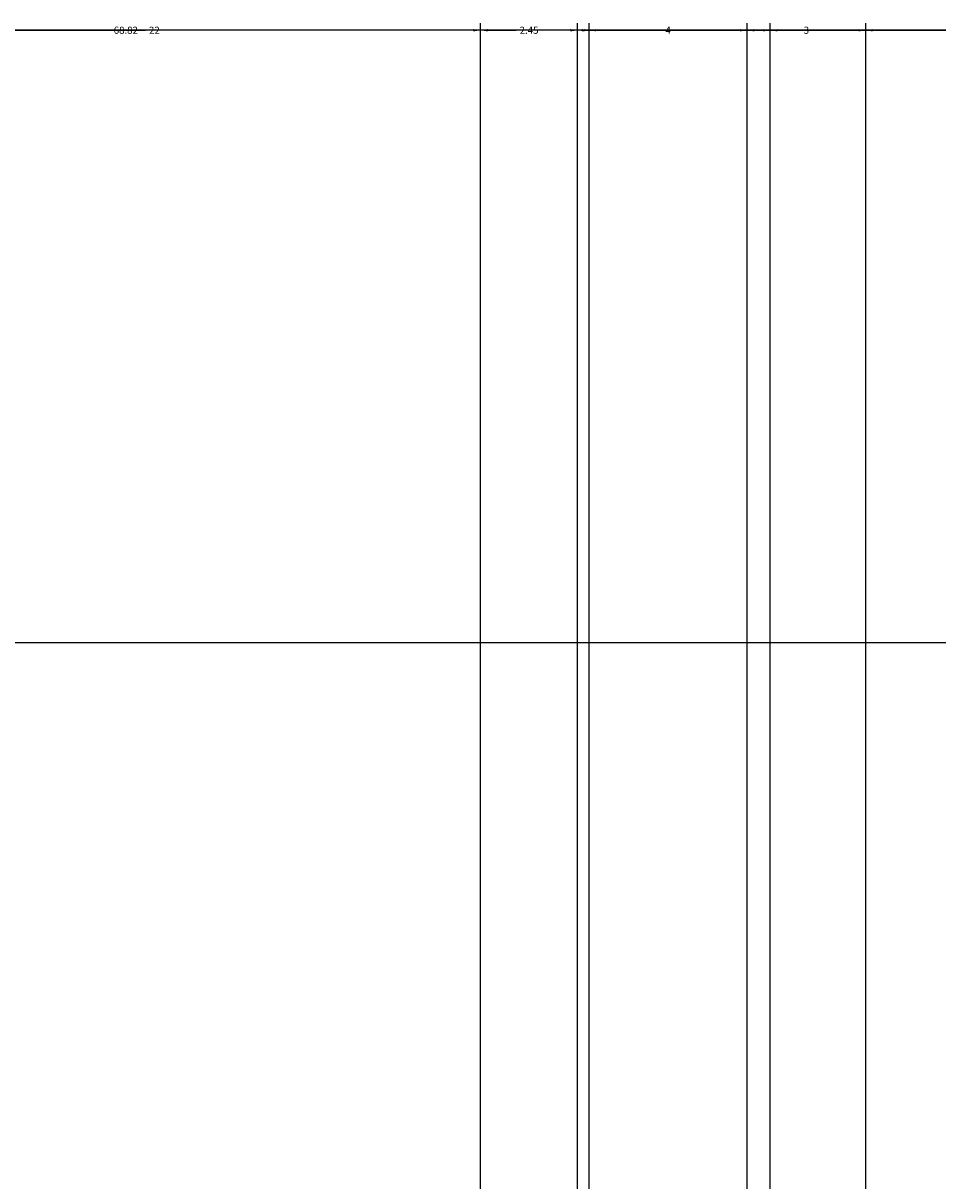
# Model space of a CAD drawing. Units: inches. Extents: x -6 to 289, y -8 to 323.
# Tile 91 of 107: x 150 to 173, y 294 to 323. Entities that reach past the tile are written whole.
import ezdxf

# ---------------------------------------------------------------- set-up
doc = ezdxf.new("R2010")
doc.units = ezdxf.units.IN
doc.header["$MEASUREMENT"] = 0
doc.layers.add('A-ANNO-DIMS', color=2, linetype='Continuous', lineweight=18)
doc.styles.get("Standard").update_dxf_attribs({"font": 'arial.ttf'})
doc.dimstyles.get("Standard").update_dxf_attribs({"dimtxt": 0.18, "dimasz": 0.18, "dimexe": 0.18, "dimexo": 0.0625, "dimgap": 0.09, "dimtad": 0, "dimtih": 1, "dimtoh": 1, "dimdec": 4, "dimzin": 0, "dimdsep": 46, "dimtxsty": 'Standard', "dimcen": 0.09, "dimadec": 0, "dimazin": 0, "dimtfac": 1, "dimtdec": 4, "dimtofl": 0, "dimtmove": 0, "dimatfit": 3, "dimfxl": 1, "dimtolj": 1, "dimtzin": 0, "dimarcsym": 0})

# ---------------------------------------------------------------- blocks, each defined once
blk = doc.blocks.new('*D11')
at = {"layer": 'A-ANNO-DIMS', "color": 0, "lineweight": -2, "transparency": 16777216}
for p, q in [((126.883, 226.717), (126.883, 322.969)), ((168.883, 226.717), (168.883, 322.969)), ((127.063, 322.789), (147.662, 322.789)), ((168.703, 322.789), (148.105, 322.789))]:
    blk.add_line(p, q, dxfattribs=at)
at = {"layer": 'A-ANNO-DIMS', "color": 0, "transparency": 16777216}
for points in [[(127.063, 322.819), (127.063, 322.759), (126.883, 322.789)], [(168.703, 322.819), (168.703, 322.759), (168.883, 322.789)]]:
    blk.add_solid(points, dxfattribs=at)
at = {"layer": 'Defpoints', "color": 0, "transparency": 16777216}
for p in [(168.883, 322.789), (126.883, 226.654), (168.883, 226.654)]:
    blk.add_point(p, dxfattribs=at)
at = {"layer": 'A-ANNO-DIMS', "color": 0, "transparency": 16777216, "insert": (147.883, 322.789), "char_height": 0.18, "attachment_point": 5}
blk.add_mtext('\\A1;42', dxfattribs=at)
blk = doc.blocks.new('*D12')
at = {"layer": 'A-ANNO-DIMS', "color": 0, "lineweight": -2, "transparency": 16777216}
for p, q in [((168.883, 226.717), (168.883, 322.969)), ((188.292, 226.951), (188.292, 322.969)), ((169.063, 322.789), (178.22, 322.789)), ((188.112, 322.789), (178.955, 322.789))]:
    blk.add_line(p, q, dxfattribs=at)
at = {"layer": 'A-ANNO-DIMS', "color": 0, "transparency": 16777216}
for points in [[(169.063, 322.819), (169.063, 322.759), (168.883, 322.789)], [(188.112, 322.819), (188.112, 322.759), (188.292, 322.789)]]:
    blk.add_solid(points, dxfattribs=at)
at = {"layer": 'Defpoints', "color": 0, "transparency": 16777216}
for p in [(188.292, 322.789), (188.292, 226.889), (168.883, 226.654)]:
    blk.add_point(p, dxfattribs=at)
at = {"layer": 'A-ANNO-DIMS', "color": 0, "transparency": 16777216, "insert": (178.588, 322.789), "char_height": 0.18, "attachment_point": 5}
blk.add_mtext('\\A1;19.41', dxfattribs=at)
blk = doc.blocks.new('*D27')
at = {"layer": 'A-ANNO-DIMS', "color": 0, "lineweight": -2, "transparency": 16777216}
for p, q in [((19.226, 307.289), (288.653, 307.289)), ((288.473, 307.109), (288.473, 277.471)), ((288.473, 247.469), (288.473, 277.107)), ((247.226, 247.289), (288.653, 247.289))]:
    blk.add_line(p, q, dxfattribs=at)
at = {"layer": 'A-ANNO-DIMS', "color": 0, "transparency": 16777216}
for points in [[(288.443, 307.109), (288.503, 307.109), (288.473, 307.289)], [(288.443, 247.469), (288.503, 247.469), (288.473, 247.289)]]:
    blk.add_solid(points, dxfattribs=at)
at = {"layer": 'Defpoints', "color": 0, "transparency": 16777216}
for p in [(19.164, 307.289), (288.473, 307.289), (247.164, 247.289)]:
    blk.add_point(p, dxfattribs=at)
at = {"layer": 'A-ANNO-DIMS', "color": 0, "transparency": 16777216, "insert": (288.473, 277.289), "char_height": 0.18, "attachment_point": 5}
blk.add_mtext('\\A1;60', dxfattribs=at)
blk = doc.blocks.new('*D76')
at = {"layer": 'A-ANNO-DIMS', "color": 0, "lineweight": -2, "transparency": 16777216}
for p, q in [((142.296, 51.148), (142.296, 322.969)), ((164.296, 51.148), (164.296, 322.969)), ((142.476, 322.789), (153.076, 322.789)), ((164.116, 322.789), (153.516, 322.789))]:
    blk.add_line(p, q, dxfattribs=at)
at = {"layer": 'A-ANNO-DIMS', "color": 0, "transparency": 16777216}
for points in [[(142.476, 322.819), (142.476, 322.759), (142.296, 322.789)], [(164.116, 322.819), (164.116, 322.759), (164.296, 322.789)]]:
    blk.add_solid(points, dxfattribs=at)
at = {"layer": 'Defpoints', "color": 0, "transparency": 16777216}
for p in [(164.296, 322.789), (142.296, 51.085), (164.296, 51.085)]:
    blk.add_point(p, dxfattribs=at)
at = {"layer": 'A-ANNO-DIMS', "color": 0, "transparency": 16777216, "insert": (153.296, 322.789), "char_height": 0.18, "attachment_point": 5}
blk.add_mtext('\\A1;22', dxfattribs=at)
blk = doc.blocks.new('*D77')
at = {"layer": 'A-ANNO-DIMS', "color": 0, "lineweight": -2, "transparency": 16777216}
for p, q in [((164.296, 51.148), (164.296, 322.969)), ((168.296, 51.148), (168.296, 322.969)), ((164.476, 322.789), (166.144, 322.789)), ((168.116, 322.789), (166.448, 322.789))]:
    blk.add_line(p, q, dxfattribs=at)
at = {"layer": 'A-ANNO-DIMS', "color": 0, "transparency": 16777216}
for points in [[(164.476, 322.819), (164.476, 322.759), (164.296, 322.789)], [(168.116, 322.819), (168.116, 322.759), (168.296, 322.789)]]:
    blk.add_solid(points, dxfattribs=at)
at = {"layer": 'Defpoints', "color": 0, "transparency": 16777216}
for p in [(168.296, 322.789), (164.296, 51.085), (168.296, 51.085)]:
    blk.add_point(p, dxfattribs=at)
at = {"layer": 'A-ANNO-DIMS', "color": 0, "transparency": 16777216, "insert": (166.296, 322.789), "char_height": 0.18, "attachment_point": 5}
blk.add_mtext('\\A1;4', dxfattribs=at)
blk = doc.blocks.new('*D78')
at = {"layer": 'A-ANNO-DIMS', "color": 0, "lineweight": -2, "transparency": 16777216}
for p, q in [((168.296, 51.148), (168.296, 322.969)), ((171.296, 51.148), (171.296, 322.969)), ((168.476, 322.789), (169.647, 322.789)), ((171.116, 322.789), (169.945, 322.789))]:
    blk.add_line(p, q, dxfattribs=at)
at = {"layer": 'A-ANNO-DIMS', "color": 0, "transparency": 16777216}
for points in [[(168.476, 322.819), (168.476, 322.759), (168.296, 322.789)], [(171.116, 322.819), (171.116, 322.759), (171.296, 322.789)]]:
    blk.add_solid(points, dxfattribs=at)
at = {"layer": 'Defpoints', "color": 0, "transparency": 16777216}
for p in [(171.296, 322.789), (168.296, 51.085), (171.296, 51.085)]:
    blk.add_point(p, dxfattribs=at)
at = {"layer": 'A-ANNO-DIMS', "color": 0, "transparency": 16777216, "insert": (169.796, 322.789), "char_height": 0.18, "attachment_point": 5}
blk.add_mtext('\\A1;3', dxfattribs=at)
blk = doc.blocks.new('*D79')
at = {"layer": 'A-ANNO-DIMS', "color": 0, "lineweight": -2, "transparency": 16777216}
for p, q in [((171.296, 118.033), (171.296, 322.969)), ((188.292, 116.842), (188.292, 322.969)), ((171.476, 322.789), (179.339, 322.789)), ((188.112, 322.789), (180.249, 322.789))]:
    blk.add_line(p, q, dxfattribs=at)
at = {"layer": 'A-ANNO-DIMS', "color": 0, "transparency": 16777216}
for points in [[(171.476, 322.819), (171.476, 322.759), (171.296, 322.789)], [(188.112, 322.819), (188.112, 322.759), (188.292, 322.789)]]:
    blk.add_solid(points, dxfattribs=at)
at = {"layer": 'Defpoints', "color": 0, "transparency": 16777216}
for p in [(188.292, 322.789), (171.296, 117.971), (188.292, 116.779)]:
    blk.add_point(p, dxfattribs=at)
at = {"layer": 'A-ANNO-DIMS', "color": 0, "transparency": 16777216, "insert": (179.794, 322.789), "char_height": 0.18, "attachment_point": 5}
blk.add_mtext('\\A1;16.996', dxfattribs=at)
blk = doc.blocks.new('*D94')
at = {"layer": 'A-ANNO-DIMS', "color": 0, "lineweight": -2, "transparency": 16777216}
for p, q in [((118.164, 159.411), (118.164, 322.969)), ((161.552, 159.411), (161.552, 322.969)), ((118.344, 322.789), (139.46, 322.789)), ((161.372, 322.789), (140.256, 322.789))]:
    blk.add_line(p, q, dxfattribs=at)
at = {"layer": 'A-ANNO-DIMS', "color": 0, "transparency": 16777216}
for points in [[(118.344, 322.819), (118.344, 322.759), (118.164, 322.789)], [(161.372, 322.819), (161.372, 322.759), (161.552, 322.789)]]:
    blk.add_solid(points, dxfattribs=at)
at = {"layer": 'Defpoints', "color": 0, "transparency": 16777216}
for p in [(161.552, 322.789), (118.164, 159.348), (161.552, 159.348)]:
    blk.add_point(p, dxfattribs=at)
at = {"layer": 'A-ANNO-DIMS', "color": 0, "transparency": 16777216, "insert": (139.858, 322.789), "char_height": 0.18, "attachment_point": 5}
blk.add_mtext('\\A1;43.39', dxfattribs=at)
blk = doc.blocks.new('*D95')
at = {"layer": 'A-ANNO-DIMS', "color": 0, "lineweight": -2, "transparency": 16777216}
for p, q in [((161.552, 159.411), (161.552, 322.969)), ((164.004, 159.411), (164.004, 322.969)), ((161.732, 322.789), (162.452, 322.789)), ((163.824, 322.789), (163.104, 322.789))]:
    blk.add_line(p, q, dxfattribs=at)
at = {"layer": 'A-ANNO-DIMS', "color": 0, "transparency": 16777216}
for points in [[(161.732, 322.819), (161.732, 322.759), (161.552, 322.789)], [(163.824, 322.819), (163.824, 322.759), (164.004, 322.789)]]:
    blk.add_solid(points, dxfattribs=at)
at = {"layer": 'Defpoints', "color": 0, "transparency": 16777216}
for p in [(164.004, 322.789), (161.552, 159.348), (164.004, 159.348)]:
    blk.add_point(p, dxfattribs=at)
at = {"layer": 'A-ANNO-DIMS', "color": 0, "transparency": 16777216, "insert": (162.778, 322.789), "char_height": 0.18, "attachment_point": 5}
blk.add_mtext('\\A1;2.45', dxfattribs=at)
blk = doc.blocks.new('*D96')
at = {"layer": 'A-ANNO-DIMS', "color": 0, "lineweight": -2, "transparency": 16777216}
for p, q in [((164.004, 159.411), (164.004, 322.969)), ((200.616, 159.411), (200.616, 322.969)), ((164.184, 322.789), (181.934, 322.789)), ((200.436, 322.789), (182.686, 322.789))]:
    blk.add_line(p, q, dxfattribs=at)
at = {"layer": 'A-ANNO-DIMS', "color": 0, "transparency": 16777216}
for points in [[(164.184, 322.819), (164.184, 322.759), (164.004, 322.789)], [(200.436, 322.819), (200.436, 322.759), (200.616, 322.789)]]:
    blk.add_solid(points, dxfattribs=at)
at = {"layer": 'Defpoints', "color": 0, "transparency": 16777216}
for p in [(200.616, 322.789), (164.004, 159.348), (200.616, 159.348)]:
    blk.add_point(p, dxfattribs=at)
at = {"layer": 'A-ANNO-DIMS', "color": 0, "transparency": 16777216, "insert": (182.31, 322.789), "char_height": 0.18, "attachment_point": 5}
blk.add_mtext('\\A1;36.61', dxfattribs=at)
blk = doc.blocks.new('*D107')
at = {"layer": 'A-ANNO-DIMS', "color": 0, "lineweight": -2, "transparency": 16777216}
for p, q in [((118.164, 293.728), (118.164, 322.969)), ((186.984, 291.541), (186.984, 322.969)), ((118.344, 322.789), (152.18, 322.789)), ((186.804, 322.789), (152.967, 322.789))]:
    blk.add_line(p, q, dxfattribs=at)
at = {"layer": 'A-ANNO-DIMS', "color": 0, "transparency": 16777216}
for points in [[(118.344, 322.819), (118.344, 322.759), (118.164, 322.789)], [(186.804, 322.819), (186.804, 322.759), (186.984, 322.789)]]:
    blk.add_solid(points, dxfattribs=at)
at = {"layer": 'Defpoints', "color": 0, "transparency": 16777216}
for p in [(186.984, 322.789), (118.164, 293.666), (186.984, 291.478)]:
    blk.add_point(p, dxfattribs=at)
at = {"layer": 'A-ANNO-DIMS', "color": 0, "transparency": 16777216, "insert": (152.574, 322.789), "char_height": 0.18, "attachment_point": 5}
blk.add_mtext('\\A1;68.82', dxfattribs=at)
blk = doc.blocks.new('*D118')
at = {"layer": 'A-ANNO-DIMS', "color": 0, "lineweight": -2, "transparency": 16777216}
for p, q in [((118.226, 307.289), (288.653, 307.289)), ((288.473, 307.109), (288.473, 300.659)), ((288.473, 293.846), (288.473, 300.295)), ((257.703, 293.666), (288.653, 293.666))]:
    blk.add_line(p, q, dxfattribs=at)
at = {"layer": 'A-ANNO-DIMS', "color": 0, "transparency": 16777216}
for points in [[(288.443, 307.109), (288.503, 307.109), (288.473, 307.289)], [(288.443, 293.846), (288.503, 293.846), (288.473, 293.666)]]:
    blk.add_solid(points, dxfattribs=at)
at = {"layer": 'Defpoints', "color": 0, "transparency": 16777216}
for p in [(118.164, 307.289), (288.473, 307.289), (257.641, 293.666)]:
    blk.add_point(p, dxfattribs=at)
at = {"layer": 'A-ANNO-DIMS', "color": 0, "transparency": 16777216, "insert": (288.473, 300.477), "char_height": 0.18, "attachment_point": 5}
blk.add_mtext('\\A1;13.623', dxfattribs=at)

msp = doc.modelspace()

# ---------------------------------------------------------------- dimensions: what is measured, and where the dimension line sits
at = {"layer": 'A-ANNO-DIMS'}
for base, p1, p2, override, picture, middle in [((161.5522, 322.7888), (118.1638, 159.3484), (161.5522, 159.3484), {"dimdec": 2, "dimlfac": 1, "dimrnd": 0, "dimzin": 0, "dimdsep": 46, "dimlunit": 2}, '*D94', (139.858, 322.7888)), ((186.9837, 322.7888), (118.1638, 293.6657), (186.9837, 291.4781), {"dimdec": 2, "dimlfac": 1, "dimrnd": 0, "dimzin": 0, "dimdsep": 46, "dimlunit": 2}, '*D107', (152.5737, 322.7888)), ((168.8835, 322.7888), (126.8835, 226.654), (168.8835, 226.654), {"dimdec": 0, "dimlfac": 1, "dimrnd": 0, "dimzin": 0, "dimdsep": 46, "dimlunit": 2}, '*D11', (147.8835, 322.7888)), ((164.296, 322.7888), (142.296, 51.0851), (164.296, 51.0851), {"dimdec": 0, "dimlfac": 1, "dimrnd": 0, "dimzin": 0, "dimdsep": 46, "dimlunit": 2}, '*D76', (153.296, 322.7888)), ((164.0039, 322.7888), (161.5522, 159.3484), (164.0039, 159.3484), {"dimdec": 2, "dimlfac": 1, "dimrnd": 0, "dimzin": 0, "dimdsep": 46, "dimlunit": 2}, '*D95', (162.7781, 322.7888)), ((200.6162, 322.7888), (164.0039, 159.3484), (200.6162, 159.3484), {"dimdec": 2, "dimlfac": 1, "dimrnd": 0, "dimzin": 0, "dimdsep": 46, "dimlunit": 2}, '*D96', (182.3101, 322.7888)), ((168.296, 322.7888), (164.296, 51.0851), (168.296, 51.0851), {"dimdec": 0, "dimlfac": 1, "dimrnd": 0, "dimzin": 0, "dimdsep": 46, "dimlunit": 2}, '*D77', (166.296, 322.7888)), ((171.296, 322.7888), (168.296, 51.0851), (171.296, 51.0851), {"dimdec": 0, "dimlfac": 1, "dimrnd": 0, "dimzin": 0, "dimdsep": 46, "dimlunit": 2}, '*D78', (169.796, 322.7888)), ((188.2918, 322.7888), (168.8835, 226.654), (188.2918, 226.8887), {"dimdec": 2, "dimlfac": 1, "dimrnd": 0, "dimzin": 0, "dimdsep": 46, "dimlunit": 2}, '*D12', (178.5876, 322.7888)), ((188.2918, 322.7888), (171.296, 117.9706), (188.2918, 116.7795), {"dimdec": 3, "dimlfac": 1, "dimrnd": 0, "dimzin": 0, "dimdsep": 46, "dimlunit": 2}, '*D79', (179.7939, 322.7888))]:
    dim = msp.add_linear_dim(base=base, p1=p1, p2=p2, dimstyle='Standard', override=override, dxfattribs=at)
    dim.commit()
    dim.dimension.update_dxf_attribs({"geometry": picture, "text_midpoint": middle})
for p1, p2, override, picture, middle in [((247.1638, 247.2888), (19.1638, 307.2888), {"dimdec": 0, "dimlfac": 1, "dimrnd": 0, "dimzin": 0, "dimdsep": 46, "dimlunit": 2}, '*D27', (288.4733, 277.2888)), ((257.6407, 293.6657), (118.1638, 307.2888), {"dimdec": 3, "dimlfac": 1, "dimrnd": 0, "dimzin": 0, "dimdsep": 46, "dimlunit": 2}, '*D118', (288.4733, 300.4773))]:
    dim = msp.add_linear_dim(base=(288.4733, 307.2888), p1=p1, p2=p2, angle=90, dimstyle='Standard', override=override, dxfattribs=at)
    dim.commit()
    dim.dimension.update_dxf_attribs({"geometry": picture, "text_midpoint": middle})

doc.saveas('drawing.dxf')
